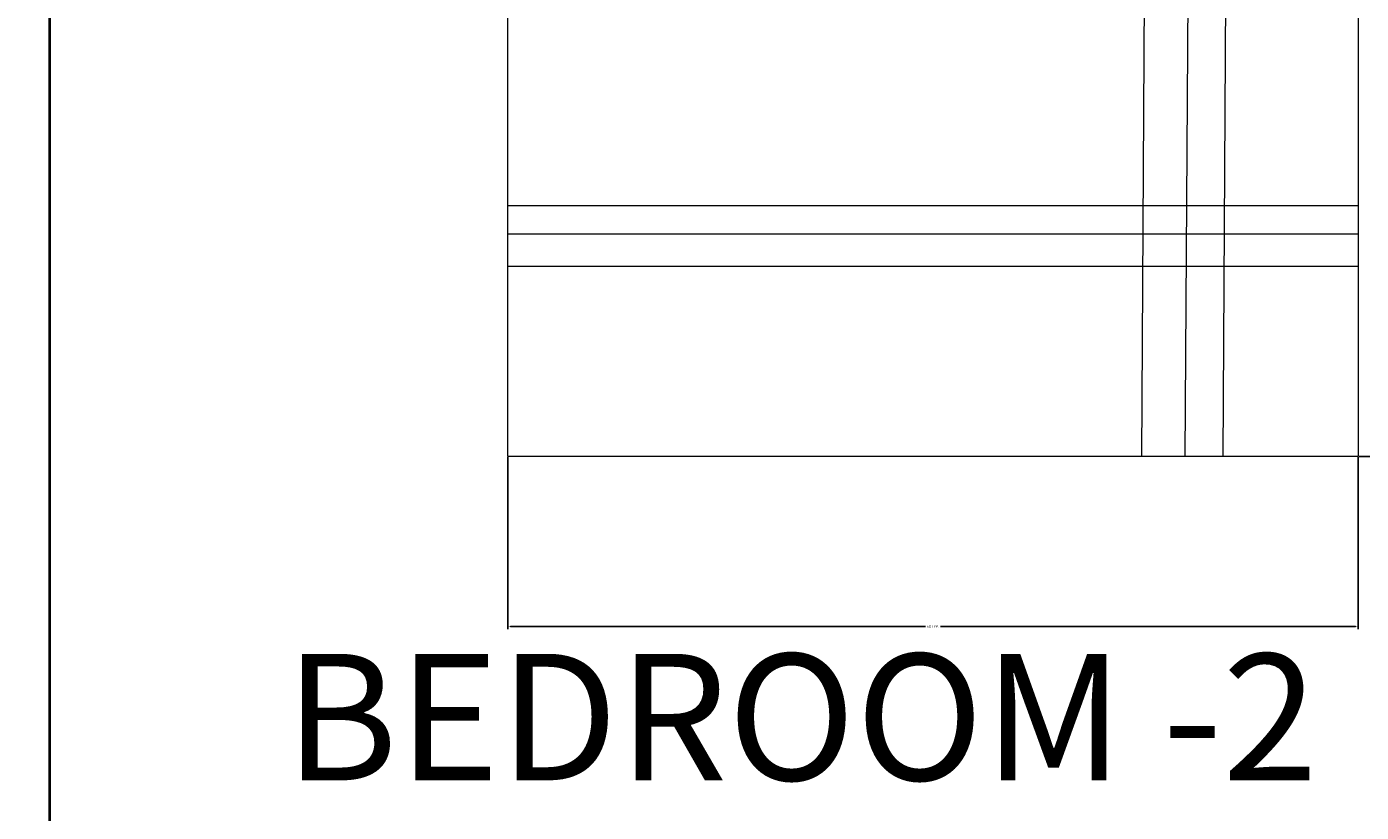
# Model space of a CAD drawing. Units: inches. Extents: x -46 to 1145, y -527 to 760.
# Tile 36 of 57: x 20 to 114, y 541 to 597. Entities that reach past the tile are written whole.
import ezdxf

# ---------------------------------------------------------------- set-up
doc = ezdxf.new("R2010")
doc.units = ezdxf.units.IN
doc.header["$MEASUREMENT"] = 0
for name, color, linetype, lineweight in [('A-ANNO-DIMS', 2, 'Continuous', 18), ('A-AREA-IDEN', 1, 'Continuous', 18), ('A-FURN', 2, 'Continuous', 13), ('WALLS', 4, 'Continuous', 40)]:
    doc.layers.add(name, color=color, linetype=linetype, lineweight=lineweight)
doc.styles.get("Standard").update_dxf_attribs({"font": 'arial.ttf'})
doc.dimstyles.get("Standard").update_dxf_attribs({"dimtxt": 0.18, "dimasz": 0.18, "dimexe": 0.18, "dimexo": 0.0625, "dimgap": 0.09, "dimtad": 0, "dimtih": 1, "dimtoh": 1, "dimdec": 0, "dimzin": 0, "dimdsep": 46, "dimlunit": 3, "dimtxsty": 'Standard', "dimcen": 0.09, "dimadec": 0, "dimazin": 0, "dimtfac": 1, "dimtdec": 0, "dimtofl": 0, "dimtmove": 0, "dimatfit": 3, "dimfxl": 1, "dimtolj": 1, "dimtzin": 0, "dimarcsym": 0})

# ---------------------------------------------------------------- blocks, each defined once
blk = doc.blocks.new('BED-QUEEN-FURNISHED')
for p, q in [((0, 0), (0, 80)), ((60, 80), (60, 0)), ((44.724, 0), (45.016, 45.372)), ((47.804, 0), (48.097, 45.499)), ((50.463, 0), (50.758, 45.907)), ((0, 17.701), (60, 17.701)), ((0, 15.692), (60, 15.692)), ((0, 13.416), (60, 13.416)), ((60, 0), (0, 0))]:
    blk.add_line(p, q)
blk = doc.blocks.new('*D652')
at = {"layer": 'A-ANNO-DIMS', "color": 0, "lineweight": -2, "transparency": 16777216}
for p, q in [((113.972, 646.503), (126.09, 646.503)), ((125.91, 646.323), (125.91, 606.691)), ((125.91, 566.683), (125.91, 606.314)), ((113.972, 566.503), (126.09, 566.503))]:
    blk.add_line(p, q, dxfattribs=at)
at = {"layer": 'A-ANNO-DIMS', "color": 0, "transparency": 16777216}
for points in [[(125.88, 646.323), (125.94, 646.323), (125.91, 646.503)], [(125.88, 566.683), (125.94, 566.683), (125.91, 566.503)]]:
    blk.add_solid(points, dxfattribs=at)
at = {"layer": 'Defpoints', "color": 0, "transparency": 16777216}
for p in [(113.91, 646.503), (125.91, 646.503), (113.91, 566.503)]:
    blk.add_point(p, dxfattribs=at)
at = {"layer": 'A-ANNO-DIMS', "color": 0, "transparency": 16777216, "insert": (125.91, 606.503), "char_height": 0.18, "attachment_point": 5}
blk.add_mtext('\\A1;QUEEN BED 80 TYP.', dxfattribs=at)
blk = doc.blocks.new('*D653')
at = {"layer": 'A-ANNO-DIMS', "color": 0, "lineweight": -2, "transparency": 16777216}
for p, q in [((53.91, 566.44), (53.91, 554.323)), ((113.91, 566.44), (113.91, 554.323)), ((54.09, 554.503), (83.381, 554.503)), ((113.73, 554.503), (84.438, 554.503))]:
    blk.add_line(p, q, dxfattribs=at)
at = {"layer": 'A-ANNO-DIMS', "color": 0, "transparency": 16777216}
for points in [[(54.09, 554.533), (54.09, 554.473), (53.91, 554.503)], [(113.73, 554.533), (113.73, 554.473), (113.91, 554.503)]]:
    blk.add_solid(points, dxfattribs=at)
at = {"layer": 'Defpoints', "color": 0, "transparency": 16777216}
for p in [(53.91, 566.503), (113.91, 566.503), (113.91, 554.503)]:
    blk.add_point(p, dxfattribs=at)
at = {"layer": 'A-ANNO-DIMS', "color": 0, "transparency": 16777216, "insert": (83.91, 554.503), "char_height": 0.18, "attachment_point": 5}
blk.add_mtext('\\A1;60 TYP.', dxfattribs=at)
blk = doc.blocks.new('*D685')
at = {"layer": 'A-ANNO-DIMS', "color": 0, "lineweight": -2, "transparency": 16777216}
for p, q in [((183.501, 700.889), (-46.216, 700.889)), ((-46.036, 700.709), (-46.036, 116.385)), ((-46.036, -468.302), (-46.036, 116.021)), ((12.501, -468.482), (-46.216, -468.482))]:
    blk.add_line(p, q, dxfattribs=at)
at = {"layer": 'A-ANNO-DIMS', "color": 0, "transparency": 16777216}
for points in [[(-46.066, 700.709), (-46.006, 700.709), (-46.036, 700.889)], [(-46.066, -468.302), (-46.006, -468.302), (-46.036, -468.482)]]:
    blk.add_solid(points, dxfattribs=at)
at = {"layer": 'Defpoints', "color": 0, "transparency": 16777216}
for p in [(-46.036, 700.889), (183.564, 700.889), (12.564, -468.482)]:
    blk.add_point(p, dxfattribs=at)
at = {"layer": 'A-ANNO-DIMS', "color": 0, "transparency": 16777216, "insert": (-46.036, 116.203), "char_height": 0.18, "attachment_point": 5}
blk.add_mtext('\\A1;1169.4', dxfattribs=at)

msp = doc.modelspace()

# ---------------------------------------------------------------- linework, layer by layer
at = {"layer": 'WALLS'}
msp.add_line((21.5637, 650.5176), (21.5637, 506.5176), dxfattribs=at)

# ---------------------------------------------------------------- block references
at = {"layer": 'A-FURN'}
msp.add_blockref('BED-QUEEN-FURNISHED', (53.91, 566.503), dxfattribs=at)

# ---------------------------------------------------------------- texts
at = {"layer": 'A-AREA-IDEN'}
msp.add_text('BEDROOM -2 ', height=8.923264, dxfattribs=at).set_placement((38.1454, 543.6508))

# ---------------------------------------------------------------- dimensions: what is measured, and where the dimension line sits
at = {"layer": 'A-ANNO-DIMS'}
dim = msp.add_linear_dim(base=(-46.0363, 700.8886), p1=(12.5637, -468.4824), p2=(183.5637, 700.8886), angle=90, dimstyle='Standard', override={"dimdec": 1, "dimlfac": 1, "dimrnd": 0, "dimzin": 0, "dimdsep": 46, "dimlunit": 2}, dxfattribs=at)
dim.commit()
dim.dimension.update_dxf_attribs({"geometry": '*D685', "text_midpoint": (-46.0363, 116.2031)})
dim = msp.add_linear_dim(base=(125.9098, 646.5029), p1=(113.9098, 566.5028), p2=(113.9098, 646.5029), angle=90, text='QUEEN BED <> TYP.', dimstyle='Standard', override={"dimdec": 0, "dimlfac": 1, "dimrnd": 0, "dimzin": 0, "dimdsep": 46, "dimlunit": 2}, dxfattribs=at)
dim.commit()
dim.dimension.update_dxf_attribs({"geometry": '*D652', "text_midpoint": (125.9098, 606.5028)})
dim = msp.add_linear_dim(base=(113.9098, 554.5028), p1=(53.9098, 566.5028), p2=(113.9098, 566.5028), text='<> TYP.', dimstyle='Standard', override={"dimdec": 0, "dimlfac": 1, "dimrnd": 0, "dimzin": 0, "dimdsep": 46, "dimlunit": 2}, dxfattribs=at)
dim.commit()
dim.dimension.update_dxf_attribs({"geometry": '*D653', "text_midpoint": (83.9098, 554.5028)})

doc.saveas('drawing.dxf')
